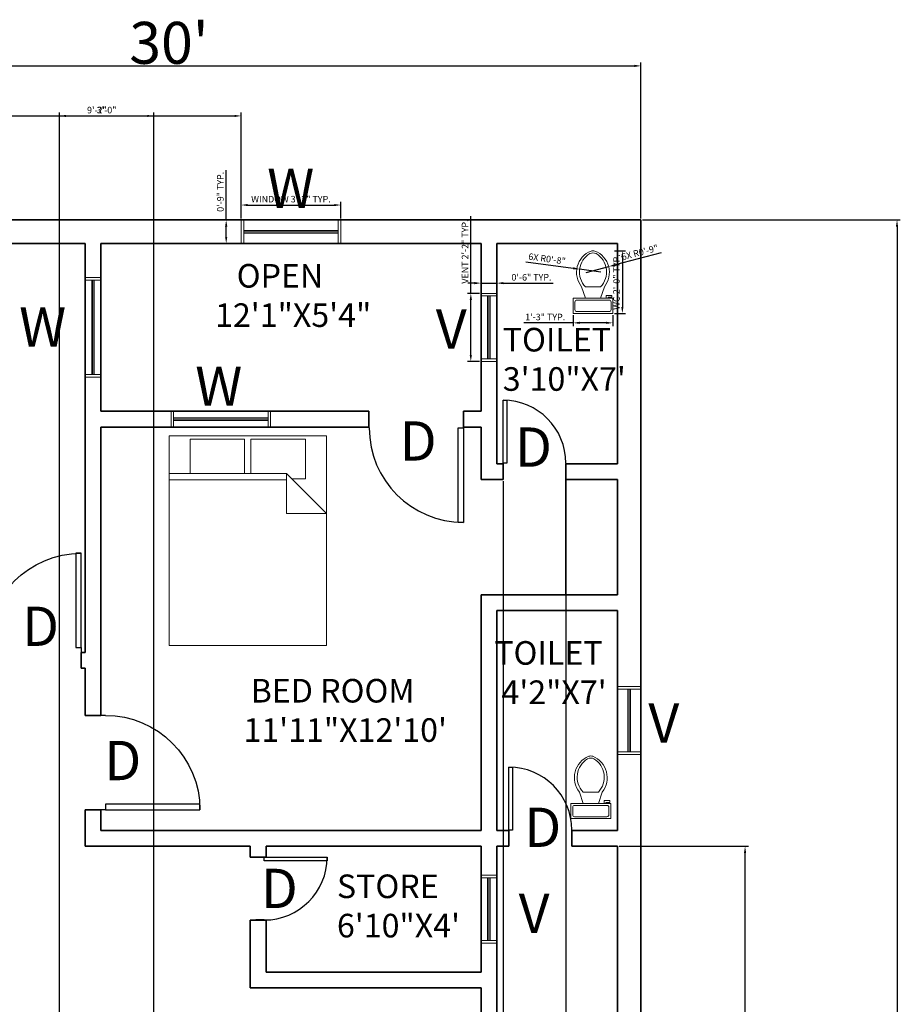
# Model space of a CAD drawing. Units: inches. Extents: x -8018 to -7514, y 7025 to 7863.
# Tile 3 of 3: x -7850 to -7514, y 7487 to 7863. Entities that reach past the tile are written whole.
import ezdxf

# ---------------------------------------------------------------- set-up
doc = ezdxf.new("R2010")
doc.units = ezdxf.units.IN
for name, color, linetype, lineweight, true_color in [('A-ANNO-DIMS', 30, 'Continuous', 18, 0xf26722), ('A-GLAZ', 240, 'Continuous', 18, 0xed1f24), ('A-WALL', 41, 'Continuous', 35, 0xf4ee51)]:
    doc.layers.add(name, color=color, linetype=linetype, lineweight=lineweight, true_color=true_color)
for name, color, linetype, lineweight in [('A-ANNO-TEXT', 7, 'Continuous', 18), ('A-AREA-IDEN', 7, 'Continuous', 18), ('A-DOOR', 4, 'Continuous', 25), ('A-FLOR-FIXT', 9, 'Continuous', 18), ('A-FURN', 9, 'Continuous', 18)]:
    doc.layers.add(name, color=color, linetype=linetype, lineweight=lineweight)
doc.styles.get("Standard").update_dxf_attribs({"font": 'arial.ttf'})
doc.dimstyles.new('ISO-25', dxfattribs={"dimtxt": 2.5, "dimasz": 2.5, "dimexe": 1.25, "dimexo": 0.625, "dimtad": 1, "dimdec": 0, "dimlunit": 3, "dimtxsty": 'Standard', "dimcen": 2.5, "dimadec": 0, "dimazin": 0, "dimtfac": 1, "dimtdec": 0, "dimtmove": 0, "dimatfit": 3, "dimfxl": 1, "dimarcsym": 0})

# ---------------------------------------------------------------- blocks, each defined once
blk = doc.blocks.new('*U8')
for p, q in [((0, 0), (0, -100)), ((750, 0), (750, -100))]:
    blk.add_line(p, q)
blk.add_lwpolyline([(0, 0), (0, 750), (43.75, 750), (43.75, 0)], close=True)
blk.add_arc((0, 0), 750, 0, 90)
blk = doc.blocks.new('Bed - Queen')
for p, q in [((0, -80.00003), (0, 0)), ((0, 0), (59.99999, 0)), ((59.99999, 0), (59.99999, -80.00003)), ((7.99999, -1.2), (28.79998, -1.2)), ((7.99999, -14.4), (7.99999, -1.2)), ((28.79998, -1.2), (28.79998, -14.4)), ((31.19999, -1.2), (51.99999, -1.2)), ((31.19999, -14.4), (31.19999, -1.2)), ((51.99999, -1.2), (51.99999, -16.4)), ((0, -14.4), (44.8, -14.4)), ((59.99999, -29.6), (44.8, -14.4)), ((44.8, -14.4), (44.8, -29.6)), ((44.8, -16.8), (0, -16.8)), ((51.99999, -16.4), (46.79936, -16.4)), ((44.8, -29.6), (59.99999, -29.6)), ((59.99999, -80.00003), (0, -80.00003))]:
    blk.add_line(p, q)
blk = doc.blocks.new('Toilet - top')
for p, q in [((9.5, -6), (9.5, -2)), ((-10, -8.5), (-8, -8.5)), ((-10, -9.5), (-10, -8.5)), ((-7, -9.5), (-10, -9.5)), ((-8, -8.5), (-8, -8)), ((-7, -8), (-7, -9.5)), ((-4, -8), (-6, -14)), ((4, -8), (6, -14)), ((4, -14), (-4, -14))]:
    blk.add_line(p, q)
blk.add_lwpolyline([(10.5, -8), (10.5, 0), (-10.5, 0), (-10.5, -8)], close=True)
for points in [[(-9.5, -2), (-9.5, -6)], [(8.5, -1), (-8.5, -1)], [(-8.5, -7), (8.5, -7)]]:
    blk.add_lwpolyline(points)
for centre, radius, start, end in [((-8.62, -1.88), 0.884, 81.8699, 188.1301), ((8.62, -1.88), 0.884, 351.8699, 98.1301), ((-8.62, -6.12), 0.884, 171.8699, 278.1301), ((8.62, -6.12), 0.884, 261.8699, 8.1301), ((3.52, -21.58), 12.17, 141.4691, 247.9714), ((4.2, -21.82), 11.33, 136.3677, 238.9468), ((-3.52, -21.58), 12.17, 292.0284, 38.5307), ((-4.2, -21.82), 11.33, 301.053, 43.6321), ((0, -27.88), 4, 245.7318, 294.2682), ((0, -29), 4, 254.8605, 285.1395)]:
    blk.add_arc(centre, radius, start, end)
blk = doc.blocks.new('*D106')
at = {"layer": 'A-ANNO-DIMS', "color": 0, "lineweight": -2, "transparency": 16777216}
for p, q in [((-7972.8, 7786.99), (-7972.8, 7846.41)), ((-7970.3, 7845.16), (-7615.3, 7845.16)), ((-7612.8, 7786.99), (-7612.8, 7846.41))]:
    blk.add_line(p, q, dxfattribs=at)
at = {"layer": 'A-ANNO-DIMS', "color": 0, "transparency": 16777216}
for points in [[(-7970.3, 7845.58), (-7970.3, 7844.75), (-7972.8, 7845.16)], [(-7615.3, 7845.58), (-7615.3, 7844.75), (-7612.8, 7845.16)]]:
    blk.add_solid(points, dxfattribs=at)
at = {"layer": 'Defpoints', "color": 0, "transparency": 16777216}
for p in [(-7612.8, 7845.16), (-7972.8, 7786.37), (-7612.8, 7786.37)]:
    blk.add_point(p, dxfattribs=at)
at = {"layer": 'A-ANNO-DIMS', "color": 0, "transparency": 16777216, "insert": (-7792.8, 7853.96), "char_height": 2.5, "attachment_point": 5}
blk.add_mtext("{\\H6.4x;30'}", dxfattribs=at)
blk = doc.blocks.new('*D107')
at = {"layer": 'A-ANNO-DIMS', "color": 0, "lineweight": -2, "transparency": 16777216}
for p, q in [((-7612.17, 7786.37), (-7513.89, 7786.37)), ((-7515.14, 7783.87), (-7515.14, 7068.87)), ((-7612.17, 7066.37), (-7513.89, 7066.37))]:
    blk.add_line(p, q, dxfattribs=at)
at = {"layer": 'A-ANNO-DIMS', "color": 0, "transparency": 16777216}
for points in [[(-7515.56, 7783.87), (-7514.73, 7783.87), (-7515.14, 7786.37)], [(-7515.56, 7068.87), (-7514.73, 7068.87), (-7515.14, 7066.37)]]:
    blk.add_solid(points, dxfattribs=at)
at = {"layer": 'Defpoints', "color": 0, "transparency": 16777216}
for p in [(-7612.8, 7786.37), (-7612.8, 7066.37), (-7515.14, 7066.37)]:
    blk.add_point(p, dxfattribs=at)
at = {"layer": 'A-ANNO-DIMS', "color": 0, "transparency": 16777216, "insert": (-7523.94, 7426.37), "char_height": 2.5, "attachment_point": 5, "rotation": 90}
blk.add_mtext("{\\H6.4x;60'}", dxfattribs=at)
blk = doc.blocks.new('VENT-24IN-6IN-WALL')
for p, q in [((0, 26), (6, 26)), ((0, 25), (6, 25)), ((2.5, 1), (2.5, 25)), ((3, 1), (3, 25)), ((3.5, 1), (3.5, 25)), ((0, 1), (6, 1)), ((0, 0), (6, 0))]:
    blk.add_line(p, q)
blk = doc.blocks.new('WINDOW-36IN-6IN-WALL')
for p, q in [((0, 38), (6, 38)), ((0, 37), (6, 37)), ((2.5, 1), (2.5, 37)), ((3, 1), (3, 37)), ((3.5, 1), (3.5, 37)), ((0, 1), (6, 1)), ((0, 0), (6, 0))]:
    blk.add_line(p, q)
blk = doc.blocks.new('WINDOW-36IN-9IN-WALL-H')
for p, q in [((0, 9), (0, 0)), ((1, 9), (1, 0)), ((37, 9), (37, 0)), ((38, 9), (38, 0)), ((1, 5), (37, 5)), ((1, 4.5), (37, 4.5)), ((1, 4), (37, 4))]:
    blk.add_line(p, q)
blk = doc.blocks.new('*D112')
at = {"layer": 'A-ANNO-DIMS', "color": 0, "lineweight": -2, "transparency": 16777216}
for p, q in [((-7677.7, 7758.37), (-7677.7, 7787.77)), ((-7674.42, 7758.37), (-7678.95, 7758.37)), ((-7677.7, 7734.87), (-7677.7, 7755.87)), ((-7674.42, 7732.37), (-7678.95, 7732.37))]:
    blk.add_line(p, q, dxfattribs=at)
at = {"layer": 'A-ANNO-DIMS', "color": 0, "transparency": 16777216}
for points in [[(-7678.12, 7755.87), (-7677.28, 7755.87), (-7677.7, 7758.37)], [(-7678.12, 7734.87), (-7677.28, 7734.87), (-7677.7, 7732.37)]]:
    blk.add_solid(points, dxfattribs=at)
at = {"layer": 'Defpoints', "color": 0, "transparency": 16777216}
for p in [(-7677.7, 7758.37), (-7673.8, 7758.37), (-7673.8, 7732.37)]:
    blk.add_point(p, dxfattribs=at)
at = {"layer": 'A-ANNO-DIMS', "color": 0, "transparency": 16777216, "insert": (-7679.58, 7774.32), "char_height": 2.5, "attachment_point": 5, "rotation": 90}
blk.add_mtext('VENT 2\'-2" TYP.', dxfattribs=at)
blk = doc.blocks.new('*D113')
at = {"layer": 'A-ANNO-DIMS', "color": 0, "lineweight": -2, "transparency": 16777216}
for p, q in [((-7676.3, 7762.27), (-7678.8, 7762.27)), ((-7673.8, 7758.99), (-7673.8, 7763.52)), ((-7673.8, 7762.27), (-7667.8, 7762.27)), ((-7667.8, 7758.99), (-7667.8, 7763.52)), ((-7665.3, 7762.27), (-7646.31, 7762.27))]:
    blk.add_line(p, q, dxfattribs=at)
at = {"layer": 'A-ANNO-DIMS', "color": 0, "transparency": 16777216}
for points in [[(-7676.3, 7762.68), (-7676.3, 7761.85), (-7673.8, 7762.27)], [(-7665.3, 7762.68), (-7665.3, 7761.85), (-7667.8, 7762.27)]]:
    blk.add_solid(points, dxfattribs=at)
at = {"layer": 'Defpoints', "color": 0, "transparency": 16777216}
for p in [(-7667.8, 7762.27), (-7673.8, 7758.37), (-7667.8, 7758.37)]:
    blk.add_point(p, dxfattribs=at)
at = {"layer": 'A-ANNO-DIMS', "color": 0, "transparency": 16777216, "insert": (-7654.56, 7764.17), "char_height": 2.5, "attachment_point": 5}
blk.add_mtext('0\'-6" TYP.', dxfattribs=at)
blk = doc.blocks.new('*D116')
at = {"layer": 'A-ANNO-DIMS', "color": 0, "lineweight": -2, "transparency": 16777216}
for p, q in [((-7765.3, 7786.99), (-7765.3, 7793.32)), ((-7727.3, 7786.99), (-7727.3, 7793.32)), ((-7762.8, 7792.07), (-7729.8, 7792.07))]:
    blk.add_line(p, q, dxfattribs=at)
at = {"layer": 'A-ANNO-DIMS', "color": 0, "transparency": 16777216}
for points in [[(-7762.8, 7792.48), (-7762.8, 7791.65), (-7765.3, 7792.07)], [(-7729.8, 7792.48), (-7729.8, 7791.65), (-7727.3, 7792.07)]]:
    blk.add_solid(points, dxfattribs=at)
at = {"layer": 'Defpoints', "color": 0, "transparency": 16777216}
for p in [(-7727.3, 7792.07), (-7765.3, 7786.37), (-7727.3, 7786.37)]:
    blk.add_point(p, dxfattribs=at)
at = {"layer": 'A-ANNO-DIMS', "color": 0, "transparency": 16777216, "insert": (-7746.3, 7793.99), "char_height": 2.5, "attachment_point": 5}
blk.add_mtext('WINDOW 3\'-2" TYP.', dxfattribs=at)
blk = doc.blocks.new('*D117')
at = {"layer": 'A-ANNO-DIMS', "color": 0, "lineweight": -2, "transparency": 16777216}
for p, q in [((-7771, 7786.37), (-7771, 7805.35)), ((-7765.92, 7786.37), (-7772.25, 7786.37)), ((-7771, 7779.87), (-7771, 7783.87)), ((-7765.92, 7777.37), (-7772.25, 7777.37))]:
    blk.add_line(p, q, dxfattribs=at)
at = {"layer": 'A-ANNO-DIMS', "color": 0, "transparency": 16777216}
for points in [[(-7771.42, 7783.87), (-7770.58, 7783.87), (-7771, 7786.37)], [(-7771.42, 7779.87), (-7770.58, 7779.87), (-7771, 7777.37)]]:
    blk.add_solid(points, dxfattribs=at)
at = {"layer": 'Defpoints', "color": 0, "transparency": 16777216}
for p in [(-7771, 7786.37), (-7765.3, 7786.37), (-7765.3, 7777.37)]:
    blk.add_point(p, dxfattribs=at)
at = {"layer": 'A-ANNO-DIMS', "color": 0, "transparency": 16777216, "insert": (-7772.9, 7797.11), "char_height": 2.5, "attachment_point": 5, "rotation": 90}
blk.add_mtext('0\'-9" TYP.', dxfattribs=at)
blk = doc.blocks.new('*D120')
at = {"layer": 'A-ANNO-DIMS', "color": 0, "lineweight": -2, "transparency": 16777216}
for p, q in [((-7622.86, 7774.65), (-7618.64, 7774.65)), ((-7619.89, 7772.15), (-7619.89, 7753.2)), ((-7622.86, 7750.7), (-7618.64, 7750.7))]:
    blk.add_line(p, q, dxfattribs=at)
at = {"layer": 'A-ANNO-DIMS', "color": 0, "transparency": 16777216}
for points in [[(-7620.31, 7772.15), (-7619.48, 7772.15), (-7619.89, 7774.65)], [(-7620.31, 7753.2), (-7619.48, 7753.2), (-7619.89, 7750.7)]]:
    blk.add_solid(points, dxfattribs=at)
at = {"layer": 'Defpoints', "color": 0, "transparency": 16777216}
for p in [(-7623.49, 7774.65), (-7623.49, 7750.7), (-7619.89, 7750.7)]:
    blk.add_point(p, dxfattribs=at)
at = {"layer": 'A-ANNO-DIMS', "color": 0, "transparency": 16777216, "insert": (-7621.81, 7762.68), "char_height": 2.5, "attachment_point": 5, "rotation": 90}
blk.add_mtext('WC 2\'-0" TYP.', dxfattribs=at)
blk = doc.blocks.new('*D121')
at = {"layer": 'A-ANNO-DIMS', "color": 0, "lineweight": -2, "transparency": 16777216}
for p, q in [((-7638.71, 7750.08), (-7638.71, 7745.86)), ((-7623.49, 7750.08), (-7623.49, 7745.86)), ((-7638.71, 7747.11), (-7657.46, 7747.11)), ((-7625.99, 7747.11), (-7636.21, 7747.11))]:
    blk.add_line(p, q, dxfattribs=at)
at = {"layer": 'A-ANNO-DIMS', "color": 0, "transparency": 16777216}
for points in [[(-7636.21, 7747.53), (-7636.21, 7746.69), (-7638.71, 7747.11)], [(-7625.99, 7747.53), (-7625.99, 7746.69), (-7623.49, 7747.11)]]:
    blk.add_solid(points, dxfattribs=at)
at = {"layer": 'Defpoints', "color": 0, "transparency": 16777216}
for p in [(-7638.71, 7750.7), (-7623.49, 7750.7), (-7638.71, 7747.11)]:
    blk.add_point(p, dxfattribs=at)
at = {"layer": 'A-ANNO-DIMS', "color": 0, "transparency": 16777216, "insert": (-7649.33, 7749.01), "char_height": 2.5, "attachment_point": 5}
blk.add_mtext('1\'-3" TYP.', dxfattribs=at)
blk = doc.blocks.new('*D132')
at = {"layer": 'A-ANNO-DIMS', "color": 0, "lineweight": -2, "transparency": 16777216}
for p, q in [((-7621.17, 7547.37), (-7571.85, 7547.37)), ((-7573.1, 7343.87), (-7573.1, 7544.87)), ((-7621.17, 7341.37), (-7571.85, 7341.37))]:
    blk.add_line(p, q, dxfattribs=at)
at = {"layer": 'A-ANNO-DIMS', "color": 0, "transparency": 16777216}
for points in [[(-7573.52, 7544.87), (-7572.68, 7544.87), (-7573.1, 7547.37)], [(-7573.52, 7343.87), (-7572.68, 7343.87), (-7573.1, 7341.37)]]:
    blk.add_solid(points, dxfattribs=at)
at = {"layer": 'Defpoints', "color": 0, "transparency": 16777216}
for p in [(-7621.8, 7547.37), (-7573.1, 7547.37), (-7621.8, 7341.37)]:
    blk.add_point(p, dxfattribs=at)
at = {"layer": 'A-ANNO-DIMS', "color": 0, "transparency": 16777216, "insert": (-7574.98, 7444.37), "char_height": 2.5, "attachment_point": 5, "rotation": 90}
blk.add_mtext('17\'-2"', dxfattribs=at)
blk = doc.blocks.new('*D133')
at = {"layer": 'A-ANNO-DIMS', "color": 0, "lineweight": -2, "transparency": 16777216}
for p, q in [((-7834.62, 7335.99), (-7834.62, 7827.32)), ((-7832.12, 7826.07), (-7801.12, 7826.07)), ((-7798.62, 7335.99), (-7798.62, 7827.32))]:
    blk.add_line(p, q, dxfattribs=at)
at = {"layer": 'A-ANNO-DIMS', "color": 0, "transparency": 16777216}
for points in [[(-7832.12, 7826.48), (-7832.12, 7825.65), (-7834.62, 7826.07)], [(-7801.12, 7826.48), (-7801.12, 7825.65), (-7798.62, 7826.07)]]:
    blk.add_solid(points, dxfattribs=at)
at = {"layer": 'Defpoints', "color": 0, "transparency": 16777216}
for p in [(-7798.62, 7826.07), (-7834.62, 7335.37), (-7798.62, 7335.37)]:
    blk.add_point(p, dxfattribs=at)
at = {"layer": 'A-ANNO-DIMS', "color": 0, "transparency": 16777216, "insert": (-7816.62, 7827.97), "char_height": 2.5, "attachment_point": 5}
blk.add_mtext('3\'-0"', dxfattribs=at)
blk = doc.blocks.new('*D137')
at = {"layer": 'A-ANNO-DIMS', "color": 0, "lineweight": -2, "transparency": 16777216}
for p, q in [((-7665.42, 7686.74), (-7665.42, 7025.42)), ((-7641.42, 7686.74), (-7641.42, 7025.42)), ((-7662.92, 7026.67), (-7643.92, 7026.67))]:
    blk.add_line(p, q, dxfattribs=at)
at = {"layer": 'A-ANNO-DIMS', "color": 0, "transparency": 16777216}
for points in [[(-7662.92, 7027.08), (-7662.92, 7026.25), (-7665.42, 7026.67)], [(-7643.92, 7027.08), (-7643.92, 7026.25), (-7641.42, 7026.67)]]:
    blk.add_solid(points, dxfattribs=at)
at = {"layer": 'Defpoints', "color": 0, "transparency": 16777216}
for p in [(-7665.42, 7687.37), (-7641.42, 7687.37), (-7641.42, 7026.67)]:
    blk.add_point(p, dxfattribs=at)
at = {"layer": 'A-ANNO-DIMS', "color": 0, "transparency": 16777216, "insert": (-7653.42, 7028.57), "char_height": 2.5, "attachment_point": 5}
blk.add_mtext('2\'-0"', dxfattribs=at)
blk = doc.blocks.new('*D139')
at = {"layer": 'A-ANNO-DIMS', "color": 0, "lineweight": -2, "transparency": 16777216}
for p, q in [((-7875.3, 7786.99), (-7875.3, 7827.32)), ((-7872.8, 7826.07), (-7767.8, 7826.07)), ((-7765.3, 7786.99), (-7765.3, 7827.32))]:
    blk.add_line(p, q, dxfattribs=at)
at = {"layer": 'A-ANNO-DIMS', "color": 0, "transparency": 16777216}
for points in [[(-7872.8, 7826.48), (-7872.8, 7825.65), (-7875.3, 7826.07)], [(-7767.8, 7826.48), (-7767.8, 7825.65), (-7765.3, 7826.07)]]:
    blk.add_solid(points, dxfattribs=at)
at = {"layer": 'Defpoints', "color": 0, "transparency": 16777216}
for p in [(-7765.3, 7826.07), (-7875.3, 7786.37), (-7765.3, 7786.37)]:
    blk.add_point(p, dxfattribs=at)
at = {"layer": 'A-ANNO-DIMS', "color": 0, "transparency": 16777216, "insert": (-7820.3, 7827.97), "char_height": 2.5, "attachment_point": 5}
blk.add_mtext('9\'-2"', dxfattribs=at)
blk = doc.blocks.new('*D142')
at = {"layer": 'A-ANNO-DIMS', "color": 0, "lineweight": -2, "transparency": 16777216}
for p, q in [((-7605.12, 7773.83), (-7622.7, 7769.22)), ((-7633.65, 7766.34), (-7625.12, 7768.58))]:
    blk.add_line(p, q, dxfattribs=at)
at = {"layer": 'A-ANNO-DIMS', "color": 0, "transparency": 16777216}
blk.add_solid([(-7622.8, 7769.62), (-7622.59, 7768.81), (-7625.12, 7768.58)], dxfattribs=at)
at = {"layer": 'Defpoints', "color": 0, "transparency": 16777216}
for p in [(-7633.65, 7766.34), (-7625.12, 7768.58)]:
    blk.add_point(p, dxfattribs=at)
at = {"layer": 'A-ANNO-DIMS', "color": 0, "transparency": 16777216, "insert": (-7613.18, 7773.68), "char_height": 2.5, "attachment_point": 5, "rotation": 14.7072}
blk.add_mtext('6X R0\'-9"', dxfattribs=at)
blk = doc.blocks.new('*D143')
at = {"layer": 'A-ANNO-DIMS', "color": 0, "lineweight": -2, "transparency": 16777216}
for p, q in [((-7656.68, 7770.37), (-7638.67, 7767.94)), ((-7628.05, 7766.51), (-7636.19, 7767.61))]:
    blk.add_line(p, q, dxfattribs=at)
at = {"layer": 'A-ANNO-DIMS', "color": 0, "transparency": 16777216}
blk.add_solid([(-7638.61, 7768.36), (-7638.72, 7767.53), (-7636.19, 7767.61)], dxfattribs=at)
at = {"layer": 'Defpoints', "color": 0, "transparency": 16777216}
for p in [(-7636.19, 7767.61), (-7628.05, 7766.51)]:
    blk.add_point(p, dxfattribs=at)
at = {"layer": 'A-ANNO-DIMS', "color": 0, "transparency": 16777216, "insert": (-7648.66, 7771.21), "char_height": 2.5, "attachment_point": 5, "rotation": 352.3271}
blk.add_mtext('6X R0\'-8"', dxfattribs=at)

msp = doc.modelspace()

# ---------------------------------------------------------------- linework, layer by layer
at = {"layer": 'A-GLAZ'}
for p, q in [((-7621.8, 7608.37), (-7612.8, 7608.37)), ((-7621.8, 7607.37), (-7612.8, 7607.37)), ((-7617.8, 7583.37), (-7617.8, 7607.37)), ((-7617.3, 7583.37), (-7617.3, 7607.37)), ((-7616.8, 7583.37), (-7616.8, 7607.37)), ((-7621.8, 7583.37), (-7612.8, 7583.37)), ((-7621.8, 7582.37), (-7612.8, 7582.37))]:
    msp.add_line(p, q, dxfattribs=at)
at = {"layer": 'A-WALL'}
for p, q in [((-7972.8, 7786.37), (-7612.8, 7786.37)), ((-7612.8, 7786.37), (-7612.8, 7066.37)), ((-7963.8, 7777.37), (-7824.8, 7777.37)), ((-7824.8, 7621.37), (-7824.8, 7777.37)), ((-7818.8, 7713.37), (-7818.8, 7777.37)), ((-7818.8, 7777.37), (-7673.8, 7777.37)), ((-7673.8, 7777.37), (-7673.8, 7713.37)), ((-7667.8, 7777.37), (-7667.8, 7693.37)), ((-7667.8, 7777.37), (-7621.8, 7777.37)), ((-7621.8, 7777.37), (-7621.8, 7693.37)), ((-7818.8, 7713.37), (-7716.55, 7713.37)), ((-7716.55, 7713.37), (-7716.55, 7707.37)), ((-7680.55, 7713.37), (-7680.55, 7707.37)), ((-7680.55, 7713.37), (-7673.8, 7713.37)), ((-7818.8, 7707.37), (-7716.55, 7707.37)), ((-7818.8, 7597.32), (-7818.8, 7707.37)), ((-7680.55, 7707.37), (-7673.8, 7707.37)), ((-7673.8, 7707.37), (-7673.8, 7687.37)), ((-7667.8, 7693.37), (-7665.42, 7693.37)), ((-7665.42, 7693.37), (-7665.42, 7687.37)), ((-7641.42, 7693.37), (-7641.42, 7687.37)), ((-7641.42, 7693.37), (-7621.8, 7693.37)), ((-7673.8, 7687.37), (-7665.42, 7687.37)), ((-7641.42, 7687.37), (-7641.42, 7643.37)), ((-7641.42, 7687.37), (-7621.8, 7687.37)), ((-7621.8, 7687.37), (-7621.8, 7643.37)), ((-7673.8, 7643.37), (-7621.8, 7643.37)), ((-7673.8, 7643.37), (-7673.8, 7553.37)), ((-7667.8, 7637.37), (-7621.8, 7637.37)), ((-7667.8, 7637.37), (-7667.8, 7553.37)), ((-7621.8, 7637.37), (-7621.8, 7553.37)), ((-7826.3, 7621.37), (-7826.3, 7615.37)), ((-7826.3, 7621.37), (-7824.8, 7621.37)), ((-7826.3, 7615.37), (-7824.8, 7615.37)), ((-7824.8, 7597.32), (-7824.8, 7615.37)), ((-7824.8, 7597.32), (-7818.8, 7597.32)), ((-7824.8, 7547.37), (-7824.8, 7561.32)), ((-7824.8, 7561.32), (-7818.8, 7561.32)), ((-7818.8, 7553.37), (-7818.8, 7561.32)), ((-7818.8, 7553.37), (-7673.8, 7553.37)), ((-7667.8, 7553.37), (-7663.16, 7553.37)), ((-7663.16, 7553.37), (-7663.16, 7547.37)), ((-7639.16, 7553.37), (-7639.16, 7547.37)), ((-7639.16, 7553.37), (-7621.8, 7553.37)), ((-7824.8, 7547.37), (-7761.8, 7547.37)), ((-7761.8, 7547.37), (-7761.8, 7543.25)), ((-7755.8, 7547.37), (-7755.8, 7543.25)), ((-7755.8, 7547.37), (-7673.8, 7547.37)), ((-7673.8, 7547.37), (-7673.8, 7499.37)), ((-7667.8, 7547.37), (-7667.8, 7452.92)), ((-7667.8, 7547.37), (-7663.16, 7547.37)), ((-7639.16, 7547.37), (-7621.8, 7547.37)), ((-7621.8, 7547.37), (-7621.8, 7341.37)), ((-7761.8, 7543.25), (-7755.8, 7543.25)), ((-7761.8, 7519.25), (-7755.8, 7519.25)), ((-7761.8, 7519.25), (-7761.8, 7493.37)), ((-7755.8, 7519.25), (-7755.8, 7499.37)), ((-7755.8, 7499.37), (-7673.8, 7499.37)), ((-7761.8, 7493.37), (-7673.8, 7493.37)), ((-7673.8, 7493.37), (-7673.8, 7452.92))]:
    msp.add_line(p, q, dxfattribs=at)

# ---------------------------------------------------------------- block references
at = {"layer": 'A-DOOR'}
for p, xscale, yscale, zscale in [((-7665.42, 7693.57), 0.0319999999999999, 0.0319999999999999, 0.0319999999999999), ((-7826.3, 7623.17), -0.0480000071715659, 0.0480000071715659, 0.0480000071715659), ((-7663.16, 7553.57), 0.0319999999999987, 0.0319999999999987, 0.0319999999999987)]:
    msp.add_blockref('*U8', p, dxfattribs=dict(at, xscale=xscale, yscale=yscale, zscale=zscale))
for p, xscale, yscale, zscale, rotation in [((-7680.44, 7706.99), 0.0479999999999998, 0.0479999999999998, 0.0479999999999998, 180), ((-7817, 7561.32), -0.048000000000001, 0.048000000000001, 0.048000000000001, 270), ((-7756.48, 7543.25), 0.0319949847760026, 0.0319949847760026, 0.0319949847760026, 270)]:
    msp.add_blockref('*U8', p, dxfattribs=dict(at, xscale=xscale, yscale=yscale, zscale=zscale, rotation=rotation))
at = {"layer": 'A-FLOR-FIXT', "xscale": 0.7246852791059593, "yscale": 0.7246852791059593, "zscale": 0.7246852791059593, "rotation": 180}
for p in [(-7631.1, 7750.7), (-7631.95, 7557.93)]:
    msp.add_blockref('Toilet - top', p, dxfattribs=at)
at = {"layer": 'A-FURN'}
msp.add_blockref('Bed - Queen', (-7792.8, 7703.97), dxfattribs=at)
at = {"layer": 'A-GLAZ'}
for name, p in [('WINDOW-36IN-9IN-WALL-H', (-7765.3, 7777.37)), ('WINDOW-36IN-6IN-WALL', (-7824.8, 7726.37)), ('VENT-24IN-6IN-WALL', (-7673.8, 7732.37))]:
    msp.add_blockref(name, p, dxfattribs=at)
for name, p, rotation in [('WINDOW-36IN-6IN-WALL', (-7792.04, 7713.37), 270.0000000000053), ('VENT-24IN-6IN-WALL', (-7667.8, 7536.37), 180)]:
    msp.add_blockref(name, p, dxfattribs=dict(at, rotation=rotation))

# ---------------------------------------------------------------- texts
at = {"layer": 'A-ANNO-TEXT', "char_height": 15, "attachment_point": 1}
for s, insert in [('{W}', (-7755.37, 7805.95)), ('{W}', (-7849.98, 7753.08)), ('{V}', (-7691.04, 7752.23)), ('{W}', (-7782.82, 7730.45)), ('{D}', (-7704.81, 7709.54)), ('{D}', (-7660.84, 7707.2)), ('{D}', (-7848.84, 7638.82)), ('{V}', (-7609.98, 7601.91)), ('{D}', (-7817.47, 7587.6)), ('{D}', (-7657.3, 7562.12)), ('{D}', (-7757.76, 7538.8)), ('{V}', (-7659.44, 7529.34))]:
    msp.add_mtext_dynamic_manual_height_columns(s, width=548.1497, gutter_width=12.5, heights=[0], dxfattribs=dict(at, insert=insert))
at = {"layer": 'A-AREA-IDEN', "char_height": 9, "attachment_point": 1}
for s, insert in [('{   OPEN\\P12\'1"X5\'4"}', (-7775.24, 7769.56)), ('{TOILET\\P3\'10"X7\'}', (-7665.51, 7745.19)), ('{ TOILET\\P  4\'2"X7\'}', (-7671.51, 7625.66)), ('{   BED ROOM\\P  11\'11"X12\'10\'}', (-7769.91, 7611.24)), ('{         STORE\\P         6\'10"X4\'}', (-7753.51, 7536.61))]:
    msp.add_mtext_dynamic_manual_height_columns(s, width=697.6004, gutter_width=12.5, heights=[0], dxfattribs=dict(at, insert=insert))

# ---------------------------------------------------------------- dimensions: what is measured, and where the dimension line sits
at = {"layer": 'A-ANNO-DIMS'}
for base, p1, p2, text, override, picture, middle in [((-7612.8, 7845.16), (-7972.8, 7786.37), (-7612.8, 7786.37), '{\\H6.4x;<>}', {"dimclrd": 0, "dimclre": 0, "dimclrt": 0}, '*D106', (-7792.8, 7853.96)), ((-7727.3, 7792.07), (-7765.3, 7786.37), (-7727.3, 7786.37), 'WINDOW <> TYP.', {"dimdec": 1, "dimlfac": 1, "dimrnd": 0, "dimzin": 1, "dimdsep": 46, "dimlunit": 4, "dimfrac": 2}, '*D116', (-7746.3, 7793.99)), ((-7667.8, 7762.27), (-7673.8, 7758.37), (-7667.8, 7758.37), '<> TYP.', {"dimdec": 1, "dimlfac": 1, "dimrnd": 0, "dimzin": 1, "dimdsep": 46, "dimlunit": 4, "dimfrac": 2}, '*D113', (-7654.56, 7764.17))]:
    dim = msp.add_linear_dim(base=base, p1=p1, p2=p2, text=text, dimstyle='ISO-25', override=override, dxfattribs=at)
    dim.commit()
    dim.dimension.update_dxf_attribs({"geometry": picture, "text_midpoint": middle})
for base, p1, p2, picture, middle in [((-7765.3, 7826.07), (-7875.3, 7786.37), (-7765.3, 7786.37), '*D139', (-7820.3, 7827.97)), ((-7798.62, 7826.07), (-7834.62, 7335.37), (-7798.62, 7335.37), '*D133', (-7816.62, 7827.97)), ((-7641.42, 7026.67), (-7665.42, 7687.37), (-7641.42, 7687.37), '*D137', (-7653.42, 7028.57))]:
    dim = msp.add_linear_dim(base=base, p1=p1, p2=p2, dimstyle='ISO-25', override={"dimdec": 1, "dimlfac": 1, "dimrnd": 0, "dimzin": 1, "dimdsep": 46, "dimlunit": 4, "dimfrac": 2}, dxfattribs=at)
    dim.commit()
    dim.dimension.update_dxf_attribs({"geometry": picture, "text_midpoint": middle})
for base, p1, p2, angle, text, override, picture, middle in [((-7771, 7786.37), (-7765.3, 7777.37), (-7765.3, 7786.37), 90, '<> TYP.', {"dimdec": 1, "dimlfac": 1, "dimrnd": 0, "dimzin": 1, "dimdsep": 46, "dimlunit": 4, "dimfrac": 2}, '*D117', (-7772.9, 7797.11)), ((-7677.7, 7758.37), (-7673.8, 7732.37), (-7673.8, 7758.37), 90, 'VENT <> TYP.', {"dimdec": 1, "dimlfac": 1, "dimrnd": 0, "dimzin": 1, "dimdsep": 46, "dimlunit": 4, "dimfrac": 2}, '*D112', (-7679.58, 7774.32)), ((-7515.14, 7066.37), (-7612.8, 7786.37), (-7612.8, 7066.37), 90, '{\\H6.4x;<>}', {"dimclrd": 0, "dimclre": 0, "dimclrt": 0}, '*D107', (-7523.94, 7426.37)), ((-7619.8945, 7750.7029), (-7623.4867, 7774.651), (-7623.4867, 7750.7029), 270, 'WC <> TYP.', {"dimdec": 1, "dimlfac": 1, "dimrnd": 0, "dimzin": 1, "dimdsep": 46, "dimlunit": 4, "dimfrac": 2}, '*D120', (-7621.8121, 7762.677)), ((-7638.71, 7747.11), (-7623.49, 7750.7), (-7638.71, 7750.7), 180, '<> TYP.', {"dimdec": 1, "dimlfac": 1, "dimrnd": 0, "dimzin": 1, "dimdsep": 46, "dimlunit": 4, "dimfrac": 2}, '*D121', (-7649.33, 7749.01))]:
    dim = msp.add_linear_dim(base=base, p1=p1, p2=p2, angle=angle, text=text, dimstyle='ISO-25', override=override, dxfattribs=at)
    dim.commit()
    dim.dimension.update_dxf_attribs({"geometry": picture, "text_midpoint": middle})
for center, mpoint, picture, middle in [((-7633.65, 7766.34), (-7625.12, 7768.58), '*D142', (-7613.18, 7773.68)), ((-7628.05, 7766.51), (-7636.19, 7767.61), '*D143', (-7648.66, 7771.21))]:
    dim = msp.add_radius_dim(center=center, mpoint=mpoint, text='6X <>', dimstyle='ISO-25', override={"dimdec": 1, "dimlfac": 1, "dimrnd": 0, "dimzin": 1, "dimdsep": 46, "dimlunit": 4, "dimfrac": 2}, dxfattribs=at)
    dim.commit()
    dim.dimension.update_dxf_attribs({"geometry": picture, "text_midpoint": middle})
dim = msp.add_linear_dim(base=(-7573.1, 7547.37), p1=(-7621.8, 7341.37), p2=(-7621.8, 7547.37), angle=90, dimstyle='ISO-25', override={"dimdec": 1, "dimlfac": 1, "dimrnd": 0, "dimzin": 1, "dimdsep": 46, "dimlunit": 4, "dimfrac": 2}, dxfattribs=at)
dim.commit()
dim.dimension.update_dxf_attribs({"geometry": '*D132', "text_midpoint": (-7574.98, 7444.37)})

doc.saveas('drawing.dxf')
